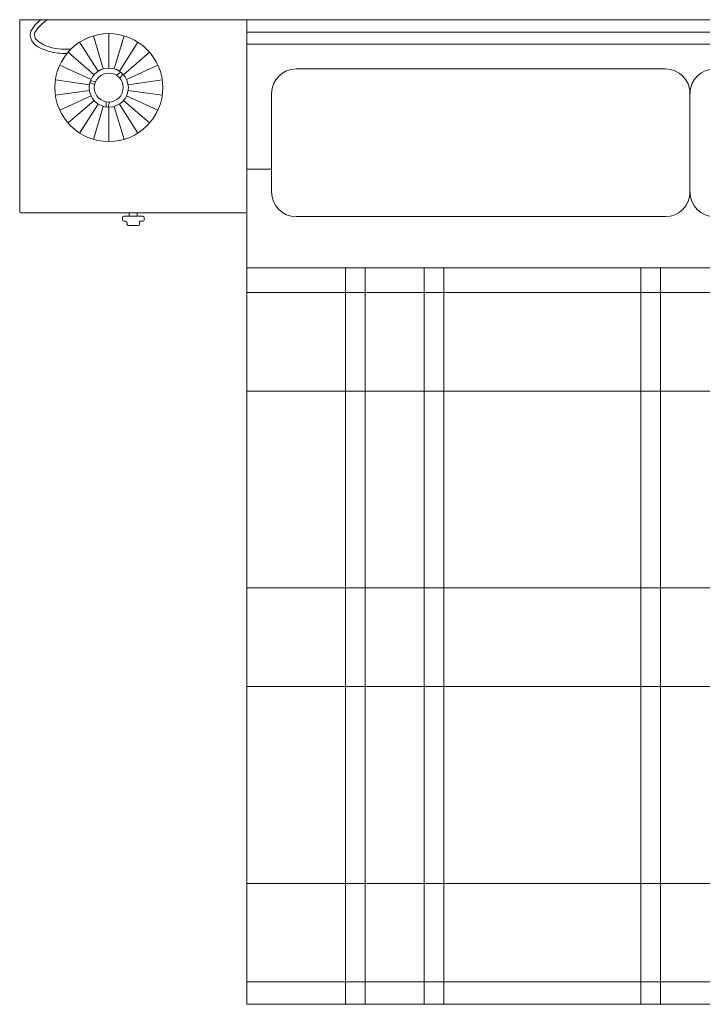
# Model space of a CAD drawing. Units: inches. Extents: x 1994 to 3075, y 3517 to 3950.
# Tile 23 of 58: x 1994.24242 to 1994.29701, y 3553.80439 to 3553.88313. Entities that reach past the tile are written whole.
import ezdxf

# ---------------------------------------------------------------- set-up
doc = ezdxf.new("R2010")
doc.units = ezdxf.units.IN
doc.layers.add('A-FURN-REFR', color=8, linetype='Continuous', lineweight=13)

msp = doc.modelspace()

# ---------------------------------------------------------------- linework, layer by layer
at = {"layer": 'A-FURN-REFR'}
for p, q in [((1994.260591, 3553.883133), (1994.242418, 3553.883133)), ((1994.242418, 3553.883133), (1994.242418, 3553.867783)), ((1994.260591, 3553.883133), (1994.242418, 3553.883133)), ((1994.331458, 3553.883133), (1994.260591, 3553.883133)), ((1994.260591, 3553.804393), (1994.260591, 3553.883133)), ((1994.260591, 3553.883133), (1994.260591, 3553.867783)), ((1994.249545, 3553.882018), (1994.249545, 3553.879265)), ((1994.249545, 3553.882018), (1994.249545, 3553.879265)), ((1994.260591, 3553.882149), (1994.331458, 3553.882149)), ((1994.247212, 3553.881332), (1994.2487, 3553.879016)), ((1994.248329, 3553.881843), (1994.249105, 3553.879201)), ((1994.250761, 3553.881843), (1994.249986, 3553.879201)), ((1994.250391, 3553.879016), (1994.251879, 3553.881332)), ((1994.260591, 3553.881165), (1994.331458, 3553.881165)), ((1994.246283, 3553.880528), (1994.248364, 3553.878725)), ((1994.250727, 3553.878725), (1994.252807, 3553.880528)), ((1994.245619, 3553.879494), (1994.248123, 3553.878351)), ((1994.250157, 3553.878685), (1994.250515, 3553.878928)), ((1994.25044, 3553.878437), (1994.250664, 3553.878793)), ((1994.250967, 3553.878351), (1994.253472, 3553.879494)), ((1994.264528, 3553.879196), (1994.294056, 3553.879196)), ((1994.245273, 3553.878315), (1994.247998, 3553.877924)), ((1994.248414, 3553.87795), (1994.248038, 3553.878116)), ((1994.248493, 3553.878186), (1994.248083, 3553.878254)), ((1994.251093, 3553.877924), (1994.253818, 3553.878315)), ((1994.245273, 3553.877087), (1994.247998, 3553.877479)), ((1994.251093, 3553.877479), (1994.253818, 3553.877087)), ((1994.26256, 3553.869354), (1994.26256, 3553.877228)), ((1994.296024, 3553.869354), (1994.296024, 3553.877228)), ((1994.245619, 3553.875908), (1994.248123, 3553.877052)), ((1994.246283, 3553.874874), (1994.248364, 3553.876677)), ((1994.247212, 3553.87407), (1994.2487, 3553.876386)), ((1994.249335, 3553.876562), (1994.249338, 3553.876152)), ((1994.249603, 3553.876544), (1994.249501, 3553.876138)), ((1994.250391, 3553.876386), (1994.251879, 3553.87407)), ((1994.250727, 3553.876677), (1994.252807, 3553.874874)), ((1994.250967, 3553.877052), (1994.253472, 3553.875908)), ((1994.249105, 3553.876201), (1994.248329, 3553.87356)), ((1994.249545, 3553.876138), (1994.249545, 3553.873385)), ((1994.249545, 3553.876138), (1994.249545, 3553.873385)), ((1994.249986, 3553.876201), (1994.250761, 3553.87356)), ((1994.260591, 3553.871179), (1994.26256, 3553.871179)), ((1994.242513, 3553.867689), (1994.260497, 3553.867689)), ((1994.250643, 3553.867324), (1994.250643, 3553.867113)), ((1994.252272, 3553.867418), (1994.250738, 3553.867418)), ((1994.250738, 3553.867019), (1994.250905, 3553.867019)), ((1994.251824, 3553.867689), (1994.251186, 3553.867689)), ((1994.251186, 3553.867689), (1994.251186, 3553.867418)), ((1994.251824, 3553.867418), (1994.251824, 3553.867689)), ((1994.25201, 3553.866767), (1994.25201, 3553.867019)), ((1994.25201, 3553.867019), (1994.252272, 3553.867019)), ((1994.252367, 3553.867113), (1994.252367, 3553.867324)), ((1994.264528, 3553.867385), (1994.294056, 3553.867385)), ((1994.251, 3553.866924), (1994.251, 3553.866767)), ((1994.251094, 3553.866672), (1994.251915, 3553.866672)), ((1994.260591, 3553.863279), (1994.331458, 3553.863279)), ((1994.268465, 3553.863279), (1994.268465, 3553.804393)), ((1994.27004, 3553.863279), (1994.27004, 3553.804393)), ((1994.274765, 3553.863279), (1994.274765, 3553.804393)), ((1994.276339, 3553.863279), (1994.276339, 3553.804393)), ((1994.292087, 3553.863279), (1994.292087, 3553.804393)), ((1994.293662, 3553.863279), (1994.293662, 3553.804393)), ((1994.260591, 3553.861311), (1994.331458, 3553.861311)), ((1994.260591, 3553.853437), (1994.331458, 3553.853437)), ((1994.260591, 3553.837689), (1994.331458, 3553.837689)), ((1994.260591, 3553.829815), (1994.331458, 3553.829815)), ((1994.260591, 3553.814067), (1994.331458, 3553.814067)), ((1994.260591, 3553.806193), (1994.331458, 3553.806193)), ((1994.331458, 3553.804393), (1994.260591, 3553.804393))]:
    msp.add_line(p, q, dxfattribs=at)
for radius in [0.004316, 0.001563, 0.001158]:
    msp.add_circle((1994.249545, 3553.877701), radius, dxfattribs=at)
for centre, radius, start, end in [((1994.264528, 3553.877228), 0.001969, 90, 180), ((1994.294056, 3553.877228), 0.001969, 0, 90), ((1994.297993, 3553.877228), 0.001969, 90, 180), ((1994.264528, 3553.869354), 0.001969, 180, 270), ((1994.294056, 3553.869354), 0.001969, 270, 0), ((1994.297993, 3553.869354), 0.001969, 180, 270), ((1994.242513, 3553.867783), 0.0000945, 180, 270), ((1994.250738, 3553.867324), 0.0000945, 90, 180), ((1994.250738, 3553.867113), 0.0000945, 180, 270), ((1994.250905, 3553.866924), 0.0000945, 0, 90), ((1994.252272, 3553.867324), 0.0000945, 0, 90), ((1994.252272, 3553.867113), 0.0000945, 270, 0), ((1994.251094, 3553.866767), 0.0000945, 180, 270), ((1994.251915, 3553.866767), 0.0000945, 270, 0)]:
    msp.add_arc(centre, radius, start, end, dxfattribs=at)
for points, knots in [([(1994.246208, 3553.880438), (1994.245735, 3553.880434), (1994.245234, 3553.880455), (1994.244167, 3553.880788), (1994.243495, 3553.88104), (1994.243134, 3553.882194), (1994.243534, 3553.882614), (1994.243979, 3553.883022), (1994.244043, 3553.883078), (1994.244107, 3553.883133)], [0.0077183, 0.0077183, 0.0077183, 0.0077183, 0.0428867, 0.0428867, 0.0785443, 0.0785443, 0.1084778, 0.1084778, 0.1132873, 0.1132873, 0.1132873, 0.1132873]), ([(1994.246508, 3553.880768), (1994.245855, 3553.880756), (1994.244833, 3553.880749), (1994.243105, 3553.881874), (1994.244049, 3553.882666), (1994.244615, 3553.883133)], [0, 0, 0, 0, 0.002019468, 0.003165929, 0.004854689, 0.004854689, 0.004854689, 0.004854689])]:
    msp.add_open_spline(points, degree=3, knots=knots, dxfattribs=at)

doc.saveas('drawing.dxf')
